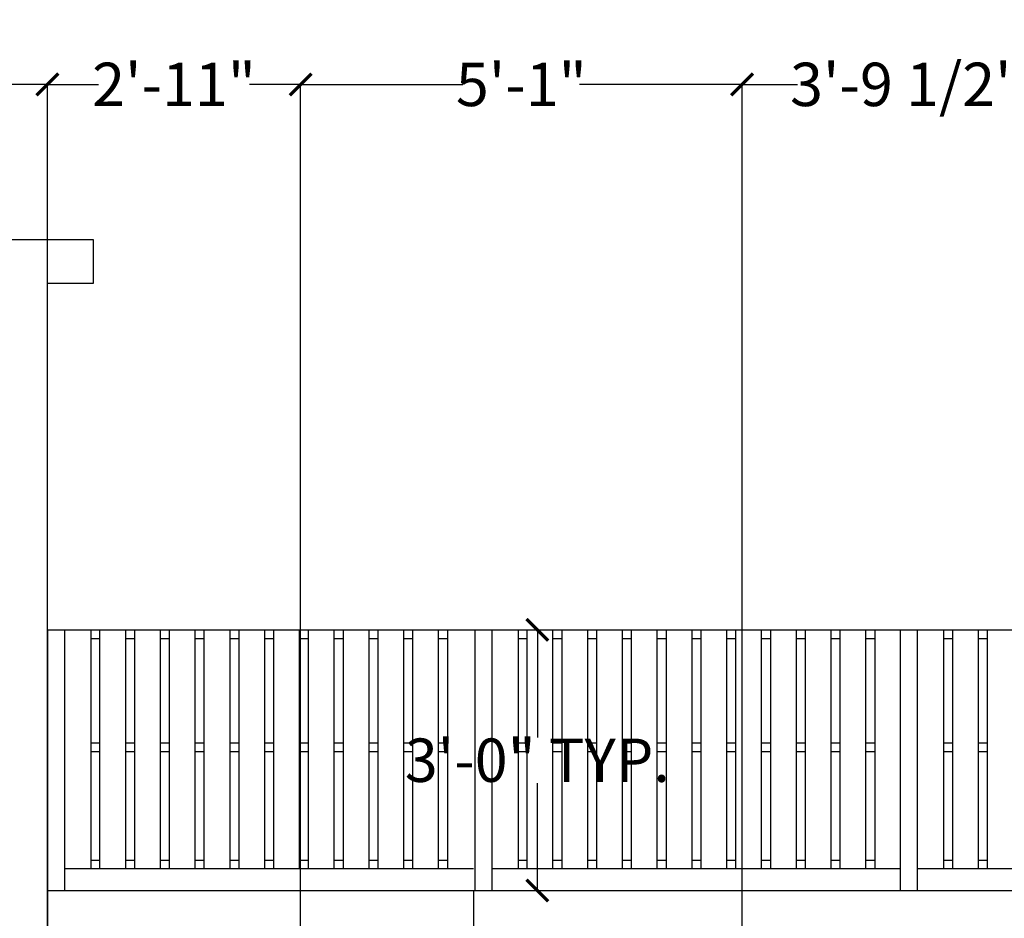
# Model space of a CAD drawing. Units: inches. Extents: x 2278 to 7495, y -71 to 1198.
# Tile 17 of 44: x 4871 to 5007, y 246 to 371. Entities that reach past the tile are written whole.
import ezdxf

# ---------------------------------------------------------------- set-up
doc = ezdxf.new("R2010")
doc.units = ezdxf.units.IN
doc.header["$MEASUREMENT"] = 0
doc.layers.add('A-ANNO-DIMS', color=2, linetype='Continuous', lineweight=18)
doc.layers.add('A-ELEV', color=7, linetype='Continuous', lineweight=25)
doc.styles.add('ATTR', font='romans.shx', dxfattribs={"width": 0.8, "height": 0.7})
doc.styles.get("Standard").update_dxf_attribs({"font": 'arial.ttf'})
doc.dimstyles.get("Standard").update_dxf_attribs({"dimtxt": 6, "dimasz": 3, "dimexe": 0.18, "dimexo": 0.0625, "dimgap": 0.09, "dimtad": 0, "dimtih": 1, "dimtoh": 1, "dimdec": 0, "dimzin": 0, "dimdsep": 46, "dimlunit": 3, "dimtxsty": 'Standard', "dimblk": 'ARCHTICK', "dimcen": 0.09, "dimadec": 0, "dimazin": 0, "dimtfac": 1, "dimtdec": 0, "dimtofl": 0, "dimtmove": 0, "dimatfit": 3, "dimfxl": 1, "dimtolj": 1, "dimtzin": 0, "dimarcsym": 0})

# ---------------------------------------------------------------- blocks, each defined once
blk = doc.blocks.new('Fence 2 EV')
for p, q in [((0, 60), (0, 0)), ((0.001, 60.008), (98.001, 60.008)), ((4, 0.002), (4, 60)), ((10, 60), (10, 5.002)), ((12, 60), (12, 5.002)), ((18, 5.002), (18, 60)), ((20, 60), (20, 5.002)), ((25.999, 5.002), (25.999, 60)), ((27.999, 60), (27.999, 5.002)), ((33.999, 5.002), (33.999, 60)), ((35.999, 60), (35.999, 5.002)), ((41.999, 5.002), (41.999, 60)), ((43.999, 60), (43.999, 5.002)), ((49.999, 5.002), (49.999, 60)), ((51.998, 60), (51.998, 5.002)), ((57.998, 5.002), (57.998, 60)), ((59.998, 60), (59.998, 5.002)), ((65.998, 5.002), (65.998, 60)), ((67.998, 60), (67.998, 5.002)), ((73.998, 5.002), (73.998, 60)), ((75.997, 60), (75.997, 5.002)), ((81.997, 5.002), (81.997, 60)), ((83.997, 60), (83.997, 5.002)), ((89.997, 5.002), (89.997, 60)), ((91.997, 60), (91.997, 5.002)), ((10, 58), (12, 58)), ((18, 58), (20, 58)), ((25.999, 58), (27.999, 58)), ((33.999, 58), (35.999, 58)), ((41.999, 58), (43.999, 58)), ((49.999, 58), (51.998, 58)), ((57.998, 58), (59.998, 58)), ((65.998, 58), (67.998, 58)), ((73.998, 58), (75.997, 58)), ((81.997, 58), (83.997, 58)), ((89.997, 58), (91.997, 58)), ((10, 34.001), (12, 34.001)), ((18, 34.001), (20, 34.001)), ((25.999, 34.001), (27.999, 34.001)), ((33.999, 34.001), (35.999, 34.001)), ((41.999, 34.001), (43.999, 34.001)), ((49.999, 34.001), (51.998, 34.001)), ((57.998, 34.001), (59.998, 34.001)), ((65.998, 34.001), (67.998, 34.001)), ((73.998, 34.001), (75.997, 34.001)), ((81.997, 34.001), (83.997, 34.001)), ((89.997, 34.001), (91.997, 34.001)), ((10, 32.001), (12, 32.001)), ((18, 32.001), (20, 32.001)), ((25.999, 32.001), (27.999, 32.001)), ((33.999, 32.001), (35.999, 32.001)), ((41.999, 32.001), (43.999, 32.001)), ((49.999, 32.001), (51.998, 32.001)), ((57.998, 32.001), (59.998, 32.001)), ((65.998, 32.001), (67.998, 32.001)), ((73.998, 32.001), (75.997, 32.001)), ((81.997, 32.001), (83.997, 32.001)), ((89.997, 32.001), (91.997, 32.001)), ((10, 7.002), (12, 7.002)), ((18, 7.002), (20, 7.002)), ((25.999, 7.002), (27.999, 7.002)), ((33.999, 7.002), (35.999, 7.002)), ((41.999, 7.002), (43.999, 7.002)), ((49.999, 7.002), (51.998, 7.002)), ((57.998, 7.002), (59.998, 7.002)), ((65.998, 7.002), (67.998, 7.002)), ((73.998, 7.002), (75.997, 7.002)), ((81.997, 7.002), (83.997, 7.002)), ((89.997, 7.002), (91.997, 7.002)), ((97.997, 5.002), (4, 5.002)), ((0, 0.002), (4, 0.002))]:
    blk.add_line(p, q)
at = {"style": 'ATTR', "width": 0.8, "flags": 9}
blk.add_attdef('ESTCODE', (0, 0), '', height=0.0196, dxfattribs=at)
blk = doc.blocks.new('_ArchTick')
at = {"color": 0, "linetype": 'ByBlock', "const_width": 0.15}
blk.add_lwpolyline([(-0.5, -0.5), (0.5, 0.5)], dxfattribs=at)
blk = doc.blocks.new('*D57')
at = {"layer": 'A-ANNO-DIMS', "color": 0, "lineweight": -2, "transparency": 16777216}
for p, q in [((4874.68, 250.19), (4874.68, 241.24)), ((4933.56, 250.19), (4933.56, 241.24)), ((4874.68, 241.42), (4933.56, 241.42)), ((4933.56, 241.42), (4936.56, 241.42))]:
    blk.add_line(p, q, dxfattribs=at)
at = {"layer": 'Defpoints', "color": 0, "transparency": 16777216}
for p in [(4874.68, 250.25), (4933.56, 250.25), (4933.56, 241.42)]:
    blk.add_point(p, dxfattribs=at)
at = {"layer": 'A-ANNO-DIMS', "color": 0, "lineweight": -2, "transparency": 16777216, "xscale": 3, "yscale": 3, "zscale": 3, "rotation": 180}
blk.add_blockref('_ArchTick', (4874.68, 241.42), dxfattribs=at)
at = {"layer": 'A-ANNO-DIMS', "color": 0, "lineweight": -2, "transparency": 16777216, "xscale": 3, "yscale": 3, "zscale": 3}
blk.add_blockref('_ArchTick', (4933.56, 241.42), dxfattribs=at)
at = {"layer": 'A-ANNO-DIMS', "color": 0, "transparency": 16777216, "insert": (4995.78, 241.42), "char_height": 6, "attachment_point": 5}
blk.add_mtext('\\A1;PARAPET RAILING 4\'-11" TYP.', dxfattribs=at)
blk = doc.blocks.new('*D58')
at = {"layer": 'A-ANNO-DIMS', "color": 0, "lineweight": -2, "transparency": 16777216}
for p, q in [((4933.62, 286.31), (4942.57, 286.31)), ((4942.39, 286.31), (4942.39, 271.43)), ((4942.39, 250.25), (4942.39, 265.12)), ((4933.62, 250.25), (4942.57, 250.25))]:
    blk.add_line(p, q, dxfattribs=at)
at = {"layer": 'Defpoints', "color": 0, "transparency": 16777216}
for p in [(4933.56, 286.31), (4942.39, 286.31), (4933.56, 250.25)]:
    blk.add_point(p, dxfattribs=at)
at = {"layer": 'A-ANNO-DIMS', "color": 0, "lineweight": -2, "transparency": 16777216, "xscale": 3, "yscale": 3, "zscale": 3}
for p, rotation in [((4942.39, 286.31), 90), ((4942.39, 250.25), 270)]:
    blk.add_blockref('_ArchTick', p, dxfattribs=dict(at, rotation=rotation))
at = {"layer": 'A-ANNO-DIMS', "color": 0, "transparency": 16777216, "insert": (4942.39, 268.28), "char_height": 6, "attachment_point": 5}
blk.add_mtext('\\A1;3\'-0" TYP.', dxfattribs=at)
blk = doc.blocks.new('*D123')
at = {"layer": 'A-ANNO-DIMS', "color": 0, "lineweight": -2, "transparency": 16777216}
for p, q in [((4736.95, 340.16), (4736.95, -23.43)), ((5145.68, -1.81), (5145.68, -23.43)), ((4736.95, -23.25), (4923.93, -23.25)), ((5145.68, -23.25), (4958.7, -23.25))]:
    blk.add_line(p, q, dxfattribs=at)
at = {"layer": 'Defpoints', "color": 0, "transparency": 16777216}
for p in [(4736.95, 340.22), (5145.68, -1.75), (5145.68, -23.25)]:
    blk.add_point(p, dxfattribs=at)
at = {"layer": 'A-ANNO-DIMS', "color": 0, "lineweight": -2, "transparency": 16777216, "xscale": 3, "yscale": 3, "zscale": 3, "rotation": 180}
blk.add_blockref('_ArchTick', (4736.95, -23.25), dxfattribs=at)
at = {"layer": 'A-ANNO-DIMS', "color": 0, "lineweight": -2, "transparency": 16777216, "xscale": 3, "yscale": 3, "zscale": 3}
blk.add_blockref('_ArchTick', (5145.68, -23.25), dxfattribs=at)
at = {"layer": 'A-ANNO-DIMS', "color": 0, "transparency": 16777216, "insert": (4941.31, -23.25), "char_height": 6, "attachment_point": 5}
blk.add_mtext('\\A1;34\'-0 1/2"', dxfattribs=at)
blk = doc.blocks.new('*D126')
at = {"layer": 'A-ANNO-DIMS', "color": 0, "lineweight": -2, "transparency": 16777216}
for p, q in [((4837.74, 313.27), (4837.74, 361.9)), ((4837.74, 361.72), (4848.14, 361.72)), ((4874.68, 361.72), (4864.27, 361.72)), ((4874.68, 99.32), (4874.68, 361.9))]:
    blk.add_line(p, q, dxfattribs=at)
at = {"layer": 'Defpoints', "color": 0, "transparency": 16777216}
for p in [(4874.68, 361.72), (4837.74, 313.21), (4874.68, 99.25)]:
    blk.add_point(p, dxfattribs=at)
at = {"layer": 'A-ANNO-DIMS', "color": 0, "lineweight": -2, "transparency": 16777216, "xscale": 3, "yscale": 3, "zscale": 3, "rotation": 180}
blk.add_blockref('_ArchTick', (4837.74, 361.72), dxfattribs=at)
at = {"layer": 'A-ANNO-DIMS', "color": 0, "lineweight": -2, "transparency": 16777216, "xscale": 3, "yscale": 3, "zscale": 3}
blk.add_blockref('_ArchTick', (4874.68, 361.72), dxfattribs=at)
at = {"layer": 'A-ANNO-DIMS', "color": 0, "transparency": 16777216, "insert": (4856.21, 361.72), "char_height": 6, "attachment_point": 5}
blk.add_mtext('\\A1;3\'-1"', dxfattribs=at)
blk = doc.blocks.new('*D127')
at = {"layer": 'A-ANNO-DIMS', "color": 0, "lineweight": -2, "transparency": 16777216}
for p, q in [((4874.68, 99.32), (4874.68, 361.9)), ((4874.68, 361.72), (4881.73, 361.72)), ((4909.68, 361.72), (4902.62, 361.72)), ((4909.68, 99.32), (4909.68, 361.9))]:
    blk.add_line(p, q, dxfattribs=at)
at = {"layer": 'Defpoints', "color": 0, "transparency": 16777216}
for p in [(4909.68, 361.72), (4874.68, 99.25), (4909.68, 99.25)]:
    blk.add_point(p, dxfattribs=at)
at = {"layer": 'A-ANNO-DIMS', "color": 0, "lineweight": -2, "transparency": 16777216, "xscale": 3, "yscale": 3, "zscale": 3, "rotation": 180}
blk.add_blockref('_ArchTick', (4874.68, 361.72), dxfattribs=at)
at = {"layer": 'A-ANNO-DIMS', "color": 0, "lineweight": -2, "transparency": 16777216, "xscale": 3, "yscale": 3, "zscale": 3}
blk.add_blockref('_ArchTick', (4909.68, 361.72), dxfattribs=at)
at = {"layer": 'A-ANNO-DIMS', "color": 0, "transparency": 16777216, "insert": (4892.18, 361.72), "char_height": 6, "attachment_point": 5}
blk.add_mtext('\\A1;2\'-11"', dxfattribs=at)
blk = doc.blocks.new('*D128')
at = {"layer": 'A-ANNO-DIMS', "color": 0, "lineweight": -2, "transparency": 16777216}
for p, q in [((4909.68, 99.32), (4909.68, 361.9)), ((4909.68, 361.72), (4932.11, 361.72)), ((4970.68, 361.72), (4948.24, 361.72)), ((4970.68, 60.78), (4970.68, 361.9))]:
    blk.add_line(p, q, dxfattribs=at)
at = {"layer": 'Defpoints', "color": 0, "transparency": 16777216}
for p in [(4970.68, 361.72), (4909.68, 99.25), (4970.68, 60.72)]:
    blk.add_point(p, dxfattribs=at)
at = {"layer": 'A-ANNO-DIMS', "color": 0, "lineweight": -2, "transparency": 16777216, "xscale": 3, "yscale": 3, "zscale": 3, "rotation": 180}
blk.add_blockref('_ArchTick', (4909.68, 361.72), dxfattribs=at)
at = {"layer": 'A-ANNO-DIMS', "color": 0, "lineweight": -2, "transparency": 16777216, "xscale": 3, "yscale": 3, "zscale": 3}
blk.add_blockref('_ArchTick', (4970.68, 361.72), dxfattribs=at)
at = {"layer": 'A-ANNO-DIMS', "color": 0, "transparency": 16777216, "insert": (4940.18, 361.72), "char_height": 6, "attachment_point": 5}
blk.add_mtext('\\A1;5\'-1"', dxfattribs=at)
blk = doc.blocks.new('*D129')
at = {"layer": 'A-ANNO-DIMS', "color": 0, "lineweight": -2, "transparency": 16777216}
for p, q in [((4970.68, 60.78), (4970.68, 361.9)), ((4970.68, 361.72), (4978.37, 361.72)), ((5016.18, 361.72), (5008.48, 361.72)), ((5016.18, 99.32), (5016.18, 361.9))]:
    blk.add_line(p, q, dxfattribs=at)
at = {"layer": 'Defpoints', "color": 0, "transparency": 16777216}
for p in [(5016.18, 361.72), (5016.18, 99.25), (4970.68, 60.72)]:
    blk.add_point(p, dxfattribs=at)
at = {"layer": 'A-ANNO-DIMS', "color": 0, "lineweight": -2, "transparency": 16777216, "xscale": 3, "yscale": 3, "zscale": 3, "rotation": 180}
blk.add_blockref('_ArchTick', (4970.68, 361.72), dxfattribs=at)
at = {"layer": 'A-ANNO-DIMS', "color": 0, "lineweight": -2, "transparency": 16777216, "xscale": 3, "yscale": 3, "zscale": 3}
blk.add_blockref('_ArchTick', (5016.18, 361.72), dxfattribs=at)
at = {"layer": 'A-ANNO-DIMS', "color": 0, "transparency": 16777216, "insert": (4993.43, 361.72), "char_height": 6, "attachment_point": 5}
blk.add_mtext('\\A1;3\'-9 1/2"', dxfattribs=at)

msp = doc.modelspace()

# ---------------------------------------------------------------- linework, layer by layer
at = {"layer": 'A-ELEV'}
for p, q in [((4881.03, 340.22), (4742.68, 340.22)), ((4881.03, 334.25), (4881.03, 340.22)), ((4874.68, 286.25), (4874.68, 334.25)), ((4874.68, 334.25), (4881.03, 334.25)), ((4874.68, 250.25), (4874.68, 286.25)), ((4874.68, 250.25), (5145.68, 250.25)), ((4874.68, 124.25), (4874.68, 250.25))]:
    msp.add_line(p, q, dxfattribs=at)

# ---------------------------------------------------------------- block references
at = {"layer": 'A-ELEV', "xscale": 0.600830084310023, "yscale": 0.600830084310023, "zscale": 0.600830084310023}
for p in [(4874.68, 250.25), (4933.74, 250.25), (4992.54, 250.25)]:
    msp.add_blockref('Fence 2 EV', p, dxfattribs=at)

# ---------------------------------------------------------------- dimensions: what is measured, and where the dimension line sits
at = {"layer": 'A-ANNO-DIMS'}
for base, p1, p2, picture, middle in [((5016.18, 361.72), (4970.68, 60.72), (5016.18, 99.25), '*D129', (4993.43, 361.72)), ((4874.68, 361.72), (4837.74, 313.21), (4874.68, 99.25), '*D126', (4856.21, 361.72)), ((4909.68, 361.72), (4874.68, 99.25), (4909.68, 99.25), '*D127', (4892.18, 361.72)), ((4970.68, 361.72), (4909.68, 99.25), (4970.68, 60.72), '*D128', (4940.18, 361.72)), ((5145.68, -23.25), (4736.95, 340.22), (5145.68, -1.75), '*D123', (4941.31, -23.25))]:
    dim = msp.add_linear_dim(base=base, p1=p1, p2=p2, dimstyle='Standard', override={"dimdec": 1, "dimlfac": 1, "dimrnd": 0, "dimzin": 1, "dimdsep": 46, "dimlunit": 4, "dimfrac": 2}, dxfattribs=at)
    dim.commit()
    dim.dimension.update_dxf_attribs({"geometry": picture, "text_midpoint": middle})
dim = msp.add_linear_dim(base=(4942.39, 286.31), p1=(4933.56, 250.25), p2=(4933.56, 286.31), angle=90, text='<> TYP.', dimstyle='Standard', override={"dimdec": 1, "dimrnd": 0, "dimzin": 1, "dimlunit": 4, "dimfrac": 2}, dxfattribs=at)
dim.commit()
dim.dimension.update_dxf_attribs({"geometry": '*D58', "text_midpoint": (4942.39, 268.28)})
dim = msp.add_linear_dim(base=(4933.56, 241.42), p1=(4874.68, 250.25), p2=(4933.56, 250.25), text='PARAPET RAILING <> TYP.', dimstyle='Standard', override={"dimdec": 1, "dimrnd": 0, "dimzin": 1, "dimlunit": 4, "dimfrac": 2}, dxfattribs=at)
dim.commit()
dim.dimension.update_dxf_attribs({"geometry": '*D57', "text_midpoint": (4995.78, 241.42)})

doc.saveas('drawing.dxf')
